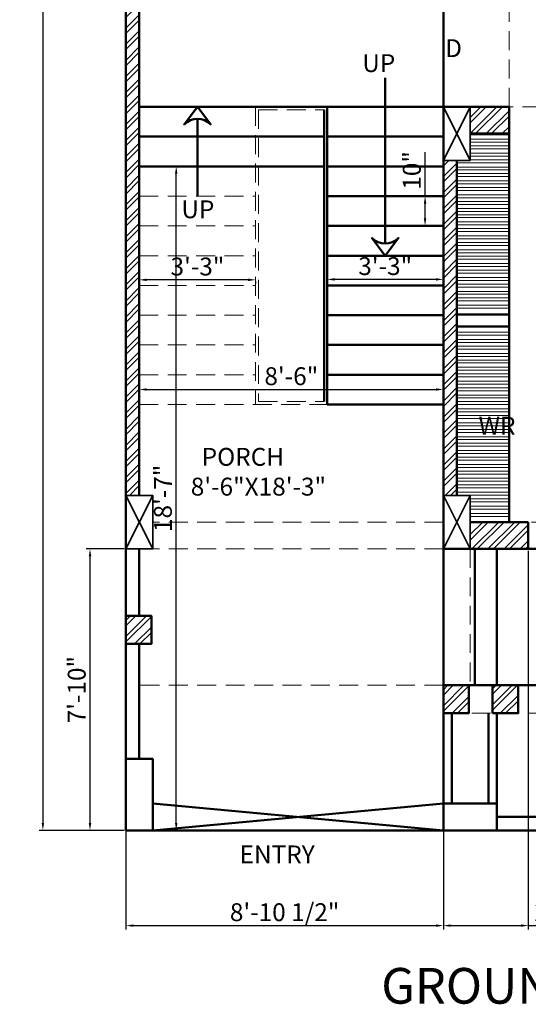
# Model space of a CAD drawing. Units: millimetres. Extents: x 67033 to 68301, y 155969 to 157209.
# Tile 1 of 17: x 67033 to 67203, y 156470 to 156800. Entities that reach past the tile are written whole.
import ezdxf

# ---------------------------------------------------------------- set-up
doc = ezdxf.new("R2010")
doc.units = ezdxf.units.MM
doc.linetypes.add('HIDDEN', pattern=[9.525, 6.35, -3.175])
for name, color, linetype, lineweight in [('A-ANNO-DIMS', 2, 'Continuous', 18), ('A-ANNO-TEXT', 7, 'Continuous', 18), ('A-AREA-IDEN', 3, 'Continuous', 18), ('A-COLS', 3, 'Continuous', 35), ('A-FLOR-OVHD', 1, 'HIDDEN', 18), ('A-FURN', 8, 'Continuous', 18), ('A-WALL', 7, 'Continuous', 50), ('A-WALL-PATT', 8, 'Continuous', 13)]:
    doc.layers.add(name, color=color, linetype=linetype, lineweight=lineweight)
doc.styles.get("Standard").update_dxf_attribs({"font": 'arial.ttf'})
doc.dimstyles.new('ISO-25', dxfattribs={"dimtxt": 6, "dimasz": 2.5, "dimexe": 1.25, "dimexo": 0.625, "dimtad": 1, "dimdec": 0, "dimlunit": 3, "dimtxsty": 'Standard', "dimcen": 2.5, "dimadec": 0, "dimazin": 0, "dimtfac": 1, "dimtdec": 0, "dimtmove": 0, "dimatfit": 3, "dimfxl": 1, "dimarcsym": 0})

# ---------------------------------------------------------------- blocks, each defined once
blk = doc.blocks.new('*D20')
at = {"layer": 'A-ANNO-DIMS', "color": 0, "lineweight": -2, "transparency": 16777216}
for p, q in [((67135.94, 156713.06), (67135.94, 156711.77)), ((67172.44, 156713.02), (67138.44, 156713.02)), ((67174.94, 156713.06), (67174.94, 156711.77))]:
    blk.add_line(p, q, dxfattribs=at)
at = {"layer": 'A-ANNO-DIMS', "color": 0, "transparency": 16777216}
for points in [[(67138.44, 156713.44), (67138.44, 156712.61), (67135.94, 156713.02)], [(67172.44, 156713.44), (67172.44, 156712.61), (67174.94, 156713.02)]]:
    blk.add_solid(points, dxfattribs=at)
at = {"layer": 'Defpoints', "color": 0, "transparency": 16777216}
for p in [(67135.94, 156713.68), (67135.94, 156713.02), (67174.94, 156713.68)]:
    blk.add_point(p, dxfattribs=at)
at = {"layer": 'A-ANNO-DIMS', "color": 0, "transparency": 16777216, "insert": (67155.44, 156716.71), "char_height": 6, "attachment_point": 5}
blk.add_mtext('3\'-3"', dxfattribs=at)
blk = doc.blocks.new('*D21')
at = {"layer": 'A-ANNO-DIMS', "color": 0, "lineweight": -2, "transparency": 16777216}
for p, q in [((67072.94, 156712.4), (67072.94, 156711.63)), ((67109.44, 156712.88), (67075.44, 156712.88)), ((67111.94, 156712.4), (67111.94, 156711.63))]:
    blk.add_line(p, q, dxfattribs=at)
at = {"layer": 'A-ANNO-DIMS', "color": 0, "transparency": 16777216}
for points in [[(67075.44, 156713.29), (67075.44, 156712.46), (67072.94, 156712.88)], [(67109.44, 156713.29), (67109.44, 156712.46), (67111.94, 156712.88)]]:
    blk.add_solid(points, dxfattribs=at)
at = {"layer": 'Defpoints', "color": 0, "transparency": 16777216}
for p in [(67072.94, 156713.02), (67072.94, 156712.88), (67111.94, 156713.02)]:
    blk.add_point(p, dxfattribs=at)
at = {"layer": 'A-ANNO-DIMS', "color": 0, "transparency": 16777216, "insert": (67092.44, 156716.57), "char_height": 6, "attachment_point": 5}
blk.add_mtext('3\'-3"', dxfattribs=at)
blk = doc.blocks.new('*D22')
at = {"layer": 'A-ANNO-DIMS', "color": 0, "lineweight": -2, "transparency": 16777216}
for p, q in [((67072.94, 156676.21), (67072.94, 156677.29)), ((67075.44, 156676.04), (67172.44, 156676.04)), ((67174.94, 156676.21), (67174.94, 156677.29))]:
    blk.add_line(p, q, dxfattribs=at)
at = {"layer": 'A-ANNO-DIMS', "color": 0, "transparency": 16777216}
for points in [[(67075.44, 156676.45), (67075.44, 156675.62), (67072.94, 156676.04)], [(67172.44, 156676.45), (67172.44, 156675.62), (67174.94, 156676.04)]]:
    blk.add_solid(points, dxfattribs=at)
at = {"layer": 'Defpoints', "color": 0, "transparency": 16777216}
for p in [(67072.94, 156675.58), (67174.94, 156676.04), (67174.94, 156675.58)]:
    blk.add_point(p, dxfattribs=at)
at = {"layer": 'A-ANNO-DIMS', "color": 0, "transparency": 16777216, "insert": (67123.94, 156679.73), "char_height": 6, "attachment_point": 5}
blk.add_mtext('8\'-6"', dxfattribs=at)
blk = doc.blocks.new('*D23')
at = {"layer": 'A-ANNO-DIMS', "color": 0, "lineweight": -2, "transparency": 16777216}
for p, q in [((67100.88, 156750.99), (67084.07, 156750.99)), ((67085.32, 156530.49), (67085.32, 156748.49)), ((67100.88, 156527.99), (67084.07, 156527.99))]:
    blk.add_line(p, q, dxfattribs=at)
at = {"layer": 'A-ANNO-DIMS', "color": 0, "transparency": 16777216}
for points in [[(67084.91, 156748.49), (67085.74, 156748.49), (67085.32, 156750.99)], [(67084.91, 156530.49), (67085.74, 156530.49), (67085.32, 156527.99)]]:
    blk.add_solid(points, dxfattribs=at)
at = {"layer": 'Defpoints', "color": 0, "transparency": 16777216}
for p in [(67085.32, 156750.99), (67101.5, 156750.99), (67101.5, 156527.99)]:
    blk.add_point(p, dxfattribs=at)
at = {"layer": 'A-ANNO-DIMS', "color": 0, "transparency": 16777216, "insert": (67081.63, 156639.49), "char_height": 6, "attachment_point": 5, "rotation": 90}
blk.add_mtext('18\'-7"', dxfattribs=at)
blk = doc.blocks.new('*D24')
at = {"layer": 'A-ANNO-DIMS', "color": 0, "lineweight": -2, "transparency": 16777216}
for p, q in [((67168.81, 156740.99), (67168.81, 156755.74)), ((67169.44, 156740.99), (67170.06, 156740.99)), ((67168.81, 156733.49), (67168.81, 156738.49)), ((67169.44, 156730.99), (67170.06, 156730.99))]:
    blk.add_line(p, q, dxfattribs=at)
at = {"layer": 'A-ANNO-DIMS', "color": 0, "transparency": 16777216}
for points in [[(67168.39, 156738.49), (67169.23, 156738.49), (67168.81, 156740.99)], [(67168.39, 156733.49), (67169.23, 156733.49), (67168.81, 156730.99)]]:
    blk.add_solid(points, dxfattribs=at)
at = {"layer": 'Defpoints', "color": 0, "transparency": 16777216}
for p in [(67168.81, 156740.99), (67168.81, 156740.99), (67168.81, 156730.99)]:
    blk.add_point(p, dxfattribs=at)
at = {"layer": 'A-ANNO-DIMS', "color": 0, "transparency": 16777216, "insert": (67165.12, 156749.62), "char_height": 6, "attachment_point": 5, "rotation": 90}
blk.add_mtext('10"', dxfattribs=at)
blk = doc.blocks.new('*D25')
at = {"layer": 'A-ANNO-DIMS', "color": 0, "lineweight": -2, "transparency": 16777216}
for p, q in [((67067.81, 156622.48), (67055.15, 156622.48)), ((67056.4, 156530.49), (67056.4, 156619.98)), ((67067.81, 156527.99), (67055.15, 156527.99))]:
    blk.add_line(p, q, dxfattribs=at)
at = {"layer": 'A-ANNO-DIMS', "color": 0, "transparency": 16777216}
for points in [[(67055.98, 156619.98), (67056.82, 156619.98), (67056.4, 156622.48)], [(67055.98, 156530.49), (67056.82, 156530.49), (67056.4, 156527.99)]]:
    blk.add_solid(points, dxfattribs=at)
at = {"layer": 'Defpoints', "color": 0, "transparency": 16777216}
for p in [(67056.4, 156622.48), (67068.44, 156622.48), (67068.44, 156527.99)]:
    blk.add_point(p, dxfattribs=at)
at = {"layer": 'A-ANNO-DIMS', "color": 0, "transparency": 16777216, "insert": (67052.71, 156575.24), "char_height": 6, "attachment_point": 5, "rotation": 90}
blk.add_mtext('7\'-10"', dxfattribs=at)
blk = doc.blocks.new('*D31')
at = {"layer": 'A-ANNO-DIMS', "color": 0, "lineweight": -2, "transparency": 16777216}
for p, q in [((67067.81, 157136.99), (67039.34, 157136.99)), ((67040.59, 157134.49), (67040.59, 156530.49)), ((67067.81, 156527.99), (67039.34, 156527.99))]:
    blk.add_line(p, q, dxfattribs=at)
at = {"layer": 'A-ANNO-DIMS', "color": 0, "transparency": 16777216}
for points in [[(67040.17, 157134.49), (67041.01, 157134.49), (67040.59, 157136.99)], [(67040.17, 156530.49), (67041.01, 156530.49), (67040.59, 156527.99)]]:
    blk.add_solid(points, dxfattribs=at)
at = {"layer": 'Defpoints', "color": 0, "transparency": 16777216}
for p in [(67068.44, 157136.99), (67040.59, 156527.99), (67068.44, 156527.99)]:
    blk.add_point(p, dxfattribs=at)
at = {"layer": 'A-ANNO-DIMS', "color": 0, "transparency": 16777216, "insert": (67036.9, 156832.49), "char_height": 6, "attachment_point": 5, "rotation": 90}
blk.add_mtext('50\'-9"', dxfattribs=at)
blk = doc.blocks.new('COLUMN-230x460')
for p, q in [((0.44, 17.99), (9.44, -0.01)), ((9.44, 17.99), (0.44, -0.01))]:
    blk.add_line(p, q)
blk.add_lwpolyline([(0.44, 17.99), (9.44, 17.99), (9.44, -0.01), (0.44, -0.01)], close=True)
blk = doc.blocks.new('*D86')
at = {"layer": 'A-ANNO-DIMS', "color": 0, "lineweight": -2, "transparency": 16777216}
for p, q in [((67068.44, 156621.85), (67068.44, 156494.74)), ((67174.94, 156621.87), (67174.94, 156494.74)), ((67070.94, 156495.99), (67172.44, 156495.99))]:
    blk.add_line(p, q, dxfattribs=at)
at = {"layer": 'A-ANNO-DIMS', "color": 0, "transparency": 16777216}
for points in [[(67070.94, 156496.41), (67070.94, 156495.58), (67068.44, 156495.99)], [(67172.44, 156496.41), (67172.44, 156495.58), (67174.94, 156495.99)]]:
    blk.add_solid(points, dxfattribs=at)
at = {"layer": 'Defpoints', "color": 0, "transparency": 16777216}
for p in [(67068.44, 156622.48), (67174.94, 156622.49), (67174.94, 156495.99)]:
    blk.add_point(p, dxfattribs=at)
at = {"layer": 'A-ANNO-DIMS', "color": 0, "transparency": 16777216, "insert": (67121.69, 156499.72), "char_height": 6, "attachment_point": 5}
blk.add_mtext('8\'-10 1/2"', dxfattribs=at)
blk = doc.blocks.new('*D87')
at = {"layer": 'A-ANNO-DIMS', "color": 0, "lineweight": -2, "transparency": 16777216}
for p, q in [((67174.94, 156621.87), (67174.94, 156494.74)), ((67203.44, 156621.87), (67203.44, 156494.74)), ((67177.44, 156495.99), (67200.94, 156495.99)), ((67203.44, 156495.99), (67237.22, 156495.99))]:
    blk.add_line(p, q, dxfattribs=at)
at = {"layer": 'A-ANNO-DIMS', "color": 0, "transparency": 16777216}
for points in [[(67177.44, 156496.41), (67177.44, 156495.58), (67174.94, 156495.99)], [(67200.94, 156496.41), (67200.94, 156495.58), (67203.44, 156495.99)]]:
    blk.add_solid(points, dxfattribs=at)
at = {"layer": 'Defpoints', "color": 0, "transparency": 16777216}
for p in [(67174.94, 156622.49), (67203.44, 156622.49), (67203.44, 156495.99)]:
    blk.add_point(p, dxfattribs=at)
at = {"layer": 'A-ANNO-DIMS', "color": 0, "transparency": 16777216, "insert": (67221.58, 156499.72), "char_height": 6, "attachment_point": 5}
blk.add_mtext('2\'-4 1/2"', dxfattribs=at)

msp = doc.modelspace()

# ---------------------------------------------------------------- hatches: boundary and pattern name
at = {"layer": 'A-WALL-PATT'}
h = msp.add_hatch(dxfattribs=at)
h.set_pattern_fill('ANSI32', color=256, scale=0.4)
h.paths.add_polyline_path([(67072.94, 156817.49), (67068.44, 156817.49), (67068.44, 156640.48), (67072.94, 156640.48)])
h = msp.add_hatch(dxfattribs=at)
h.set_pattern_fill('ANSI32', color=256, scale=0.4)
h.paths.add_polyline_path([(67196.98, 156770.99), (67183.94, 156770.99), (67183.94, 156761.99), (67196.98, 156761.99)])
h = msp.add_hatch(dxfattribs=at)
h.set_pattern_fill('ANSI32', color=256, scale=0.4)
h.paths.add_polyline_path([(67179.44, 156752.99), (67174.94, 156752.99), (67174.94, 156640.48), (67179.44, 156640.48)])
h = msp.add_hatch(dxfattribs=at)
h.set_pattern_fill('ANSI32', color=256, scale=0.4)
h.paths.add_polyline_path([(67203.44, 156631.49), (67183.94, 156631.49), (67183.94, 156622.49), (67203.44, 156622.49)])
h = msp.add_hatch(dxfattribs=at)
h.set_pattern_fill('ANSI32', color=256, scale=0.4)
h.set_pattern_definition([(45, (-106.5, 23.292), (-2.69407684, 2.69407684), []), (45, (-104.704, 23.292), (-2.69407684, 2.69407684), [])])
h.paths.add_polyline_path([(67076.99, 156600.01), (67068.44, 156600.01), (67068.44, 156590.61), (67076.99, 156590.61)])
h = msp.add_hatch(dxfattribs=at)
h.set_pattern_fill('ANSI32', color=256, scale=0.4)
h.paths.add_polyline_path([(67183.49, 156576.72), (67174.94, 156576.72), (67174.94, 156567.32), (67183.49, 156567.32)])
h = msp.add_hatch(dxfattribs=at)
h.set_pattern_fill('ANSI32', color=256, scale=0.4)
h.paths.add_polyline_path([(67200, 156576.72), (67191.45, 156576.72), (67191.45, 156567.32), (67200, 156567.32)])

# ---------------------------------------------------------------- linework, layer by layer
at = {"layer": 'A-FLOR-OVHD'}
for p, q in [((67196.98, 156770.99), (67196.98, 156817.49)), ((67111.94, 156770.99), (67111.94, 156670.99)), ((67236.44, 156770.99), (67196.98, 156770.99)), ((67112.94, 156769.99), (67112.94, 156671.99)), ((67112.94, 156769.99), (67134.94, 156769.99)), ((67072.94, 156740.99), (67111.94, 156740.99)), ((67072.94, 156730.99), (67111.94, 156730.99)), ((67072.94, 156720.99), (67111.94, 156720.99)), ((67072.94, 156710.99), (67111.94, 156710.99)), ((67072.94, 156700.99), (67111.94, 156700.99)), ((67072.94, 156690.99), (67111.94, 156690.99)), ((67072.94, 156680.99), (67111.94, 156680.99)), ((67112.94, 156671.99), (67134.94, 156671.99)), ((67072.94, 156670.99), (67135.94, 156670.99)), ((67174.94, 156631.48), (67077.44, 156631.48)), ((67239.44, 156631.49), (67203.44, 156631.49)), ((67174.94, 156622.48), (67068.44, 156622.48)), ((67183.94, 156622.48), (67183.94, 156576.72)), ((67174.94, 156576.72), (67072.94, 156576.72)), ((67174.94, 156567.32), (67302.44, 156567.32))]:
    msp.add_line(p, q, dxfattribs=at)
at = {"layer": 'A-FURN'}
for p, q in [((67183.94, 156761.54), (67196.98, 156761.54)), ((67183.94, 156760.09), (67196.98, 156760.09)), ((67183.94, 156759.09), (67196.98, 156759.09)), ((67183.94, 156757.87), (67196.98, 156757.87)), ((67183.94, 156756.87), (67196.98, 156756.87)), ((67183.94, 156755.43), (67196.98, 156755.43)), ((67183.94, 156754.43), (67196.98, 156754.43)), ((67179.44, 156752.21), (67196.98, 156752.21)), ((67179.44, 156750.77), (67196.98, 156750.77)), ((67183.83, 156753.21), (67196.98, 156753.21)), ((67179.44, 156749.77), (67196.98, 156749.77)), ((67179.44, 156748.55), (67196.98, 156748.55)), ((67179.44, 156747.55), (67196.98, 156747.55)), ((67179.44, 156746.1), (67196.98, 156746.1)), ((67179.44, 156745.1), (67196.98, 156745.1)), ((67179.44, 156743.88), (67196.98, 156743.88)), ((67179.44, 156742.88), (67196.98, 156742.88)), ((67179.44, 156741.44), (67196.98, 156741.44)), ((67179.44, 156740.44), (67196.98, 156740.44)), ((67179.44, 156739.22), (67196.98, 156739.22)), ((67179.44, 156738.22), (67196.98, 156738.22)), ((67179.44, 156736.78), (67196.98, 156736.78)), ((67179.44, 156735.78), (67196.98, 156735.78)), ((67179.44, 156734.76), (67196.98, 156734.76)), ((67179.44, 156733.76), (67196.98, 156733.76)), ((67179.44, 156732.32), (67196.98, 156732.32)), ((67179.44, 156731.32), (67196.98, 156731.32)), ((67179.44, 156730.1), (67196.98, 156730.1)), ((67179.44, 156729.1), (67196.98, 156729.1)), ((67179.44, 156727.66), (67196.98, 156727.66)), ((67179.44, 156726.66), (67196.98, 156726.66)), ((67179.44, 156725.44), (67196.98, 156725.44)), ((67179.44, 156724.44), (67196.98, 156724.44)), ((67179.44, 156722.99), (67196.98, 156722.99)), ((67179.44, 156721.99), (67196.98, 156721.99)), ((67179.44, 156720.77), (67196.98, 156720.77)), ((67179.44, 156719.77), (67196.98, 156719.77)), ((67179.44, 156718.33), (67196.98, 156718.33)), ((67179.44, 156717.33), (67196.98, 156717.33)), ((67179.44, 156716.11), (67196.98, 156716.11)), ((67179.44, 156715.11), (67196.98, 156715.11)), ((67179.44, 156713.67), (67196.98, 156713.67)), ((67179.44, 156712.67), (67196.98, 156712.67)), ((67179.44, 156711.45), (67196.98, 156711.45)), ((67179.44, 156710.45), (67196.98, 156710.45)), ((67179.44, 156709.01), (67196.98, 156709.01)), ((67179.44, 156708.01), (67196.98, 156708.01)), ((67179.44, 156706.79), (67196.98, 156706.79)), ((67179.44, 156705.79), (67196.98, 156705.79)), ((67179.44, 156704.34), (67196.98, 156704.34)), ((67179.44, 156703.34), (67196.98, 156703.34)), ((67179.44, 156695.28), (67196.98, 156695.28)), ((67179.44, 156694.28), (67196.98, 156694.28)), ((67179.44, 156692.84), (67196.98, 156692.84)), ((67179.44, 156691.84), (67196.98, 156691.84)), ((67179.44, 156690.62), (67196.98, 156690.62)), ((67179.44, 156689.62), (67196.98, 156689.62)), ((67179.44, 156688.17), (67196.98, 156688.17)), ((67179.44, 156687.17), (67196.98, 156687.17)), ((67179.44, 156685.95), (67196.98, 156685.95)), ((67179.44, 156684.95), (67196.98, 156684.95)), ((67179.44, 156683.51), (67196.98, 156683.51)), ((67179.44, 156682.51), (67196.98, 156682.51)), ((67179.44, 156681.29), (67196.98, 156681.29)), ((67179.44, 156680.29), (67196.98, 156680.29)), ((67179.44, 156678.85), (67196.98, 156678.85)), ((67179.44, 156677.85), (67196.98, 156677.85)), ((67179.44, 156676.63), (67196.98, 156676.63)), ((67179.44, 156675.63), (67196.98, 156675.63)), ((67179.44, 156674.19), (67196.98, 156674.19)), ((67179.44, 156673.19), (67196.98, 156673.19)), ((67179.44, 156671.97), (67196.98, 156671.97)), ((67179.44, 156670.97), (67196.98, 156670.97)), ((67179.44, 156669.52), (67196.98, 156669.52)), ((67179.44, 156668.52), (67196.98, 156668.52)), ((67179.44, 156667.3), (67196.98, 156667.3)), ((67179.44, 156666.3), (67196.98, 156666.3)), ((67179.44, 156664.86), (67196.98, 156664.86)), ((67179.44, 156663.86), (67196.98, 156663.86)), ((67179.44, 156662.64), (67196.98, 156662.64)), ((67179.44, 156661.64), (67196.98, 156661.64)), ((67179.44, 156660.2), (67196.98, 156660.2)), ((67179.44, 156659.2), (67196.98, 156659.2)), ((67179.44, 156657.98), (67196.98, 156657.98)), ((67179.44, 156656.98), (67196.98, 156656.98)), ((67179.44, 156655.53), (67196.98, 156655.53)), ((67179.44, 156654.53), (67196.98, 156654.53)), ((67179.44, 156653.31), (67196.98, 156653.31)), ((67179.44, 156652.31), (67196.98, 156652.31)), ((67179.44, 156650.87), (67196.98, 156650.87)), ((67179.44, 156649.87), (67196.98, 156649.87)), ((67179.44, 156648.65), (67196.98, 156648.65)), ((67179.44, 156647.65), (67196.98, 156647.65)), ((67179.44, 156646.21), (67196.98, 156646.21)), ((67179.44, 156645.21), (67196.98, 156645.21)), ((67179.44, 156643.99), (67196.98, 156643.99)), ((67179.44, 156642.99), (67196.98, 156642.99)), ((67179.44, 156641.55), (67196.98, 156641.55)), ((67179.44, 156640.55), (67196.98, 156640.55)), ((67183.94, 156639.33), (67196.98, 156639.33)), ((67183.94, 156638.33), (67196.98, 156638.33)), ((67183.94, 156636.89), (67196.98, 156636.89)), ((67183.94, 156635.89), (67196.98, 156635.89)), ((67183.94, 156634.35), (67196.98, 156634.35)), ((67183.94, 156633.35), (67196.98, 156633.35))]:
    msp.add_line(p, q, dxfattribs=at)
at = {"layer": 'A-WALL'}
for p, q in [((67068.44, 157136.99), (67068.44, 156527.99)), ((67174.94, 156821.99), (67174.94, 156622.49)), ((67072.94, 156817.49), (67072.94, 156640.48)), ((67155.44, 156725.08), (67155.44, 156780.67)), ((67072.94, 156770.99), (67174.94, 156770.99)), ((67135.94, 156770.99), (67135.94, 156670.99)), ((67174.94, 156770.99), (67196.98, 156770.99)), ((67196.98, 156770.99), (67196.98, 156631.49)), ((67134.94, 156769.99), (67134.94, 156671.99)), ((67092.44, 156740.99), (67092.44, 156766.9)), ((67072.94, 156760.99), (67134.94, 156760.99)), ((67135.94, 156760.99), (67174.94, 156760.99)), ((67183.94, 156761.99), (67196.98, 156761.99)), ((67072.94, 156750.99), (67134.94, 156750.99)), ((67135.94, 156750.99), (67174.94, 156750.99)), ((67179.44, 156752.99), (67179.44, 156640.48)), ((67135.94, 156740.99), (67174.94, 156740.99)), ((67135.94, 156730.99), (67174.94, 156730.99)), ((67135.94, 156720.99), (67174.94, 156720.99)), ((67135.94, 156710.99), (67174.94, 156710.99)), ((67135.94, 156700.99), (67174.94, 156700.99)), ((67196.98, 156701.24), (67179.44, 156701.24)), ((67196.98, 156697.24), (67179.44, 156697.24)), ((67135.94, 156690.99), (67174.94, 156690.99)), ((67135.94, 156680.99), (67174.94, 156680.99)), ((67135.94, 156670.99), (67174.94, 156670.99)), ((67183.94, 156631.49), (67203.44, 156631.49)), ((67203.44, 156631.49), (67203.44, 156622.49)), ((67072.94, 156622.48), (67072.94, 156600.01)), ((67174.94, 156622.49), (67203.44, 156622.49)), ((67174.94, 156622.48), (67174.94, 156527.99)), ((67185.55, 156622.49), (67185.55, 156576.72)), ((67192.94, 156576.72), (67192.94, 156622.49)), ((67203.44, 156622.49), (67239.44, 156622.49)), ((67072.94, 156590.61), (67072.94, 156551.99)), ((67174.94, 156576.72), (67302.44, 156576.72)), ((67177.84, 156567.32), (67177.84, 156536.99)), ((67190.04, 156567.32), (67190.04, 156536.99)), ((67192.94, 156536.99), (67192.94, 156567.32)), ((67174.94, 156536.99), (67077.44, 156527.99)), ((67174.94, 156527.99), (67077.44, 156536.99)), ((67192.94, 156532.49), (67407.44, 156532.49)), ((67068.44, 156527.99), (67407.44, 156527.99))]:
    msp.add_line(p, q, dxfattribs=at)
for points in [[(67092.44, 156770.99), (67096.9, 156765.06, 0.414166), (67087.98, 156765.06)], [(67155.44, 156720.99), (67150.98, 156726.93, 0.414166), (67159.9, 156726.93)]]:
    msp.add_lwpolyline(points, format="xyb", close=True, dxfattribs=at)
for points in [[(67068.44, 156590.61), (67076.99, 156590.61), (67076.99, 156600.01), (67068.44, 156600.01)], [(67174.94, 156567.32), (67183.49, 156567.32), (67183.49, 156576.72), (67174.94, 156576.72)], [(67191.45, 156567.32), (67200, 156567.32), (67200, 156576.72), (67191.45, 156576.72)], [(67068.44, 156527.99), (67077.44, 156527.99), (67077.44, 156551.99), (67068.44, 156551.99)], [(67174.94, 156527.99), (67192.94, 156527.99), (67192.94, 156536.99), (67174.94, 156536.99)]]:
    msp.add_lwpolyline(points, close=True, dxfattribs=at)

# ---------------------------------------------------------------- block references
at = {"layer": 'A-COLS'}
for p in [(67174.5, 156753), (67068, 156622.49)]:
    msp.add_blockref('COLUMN-230x460', p, dxfattribs=at)
at = {"layer": 'A-COLS', "extrusion": (0, 0, -1), "zscale": -1, "rotation": 180.0076170266062}
msp.add_blockref('COLUMN-230x460', (-67174.5, 156640.48), dxfattribs=at)

# ---------------------------------------------------------------- texts
at = {"layer": 'A-ANNO-TEXT', "attachment_point": 1}
for s, width, insert, char_height in [('   D', 19.5287, (67170.06, 156793.68), 6), (' UP', 19.5287, (67145.89, 156788.65), 6), (' UP', 19.5287, (67085.21, 156739.56), 6), ('   WR', 19.5287, (67181.25, 156666.88), 6), ('GROUND FLOOR PLAN', 203.6887, (67154.11, 156481.77), 12)]:
    msp.add_mtext_dynamic_manual_height_columns(s, width=width, gutter_width=12.5, heights=[0], dxfattribs=dict(at, insert=insert, char_height=char_height))
at = {"layer": 'A-AREA-IDEN', "char_height": 6, "attachment_point": 1}
for s, width, insert in [('       PORCH\\P     8\'-6"X18\'-3"', 75.351, (67081.03, 156656.42)), ('    ENTRY', 59.4046, (67099.26, 156522.9))]:
    msp.add_mtext_dynamic_manual_height_columns(s, width=width, gutter_width=12.5, heights=[0], dxfattribs=dict(at, insert=insert))

# ---------------------------------------------------------------- dimensions: what is measured, and where the dimension line sits
at = {"layer": 'A-ANNO-DIMS'}
for base, p1, p2, picture, middle in [((67040.59, 156527.99), (67068.44, 157136.99), (67068.44, 156527.99), '*D31', (67036.9, 156832.49)), ((67168.81, 156740.99), (67168.81, 156730.99), (67168.81, 156740.99), '*D24', (67165.12, 156749.62)), ((67085.32, 156750.99), (67101.5, 156527.99), (67101.5, 156750.99), '*D23', (67081.63, 156639.49)), ((67056.4, 156622.48), (67068.44, 156527.99), (67068.44, 156622.48), '*D25', (67052.71, 156575.24))]:
    dim = msp.add_linear_dim(base=base, p1=p1, p2=p2, angle=90, dimstyle='ISO-25', override={"dimclrd": 0, "dimclre": 0, "dimclrt": 0}, dxfattribs=at)
    dim.commit()
    dim.dimension.update_dxf_attribs({"geometry": picture, "text_midpoint": middle})
for base, p1, p2, override, picture, middle in [((67135.94, 156713.02), (67174.94, 156713.68), (67135.94, 156713.68), {"dimclrd": 0, "dimclre": 0, "dimclrt": 0}, '*D20', (67155.44, 156716.71)), ((67072.94, 156712.88), (67111.94, 156713.02), (67072.94, 156713.02), {"dimclrd": 0, "dimclre": 0, "dimclrt": 0}, '*D21', (67092.44, 156716.57)), ((67174.94, 156676.04), (67072.94, 156675.58), (67174.94, 156675.58), {"dimclrd": 0, "dimclre": 0, "dimclrt": 0}, '*D22', (67123.94, 156679.73)), ((67174.94, 156495.99), (67068.44, 156622.48), (67174.94, 156622.49), {"dimdec": 1, "dimlfac": 1, "dimrnd": 0, "dimzin": 1, "dimdsep": 46, "dimlunit": 4, "dimfrac": 2}, '*D86', (67121.69, 156499.72)), ((67203.44, 156495.99), (67174.94, 156622.49), (67203.44, 156622.49), {"dimdec": 1, "dimlfac": 1, "dimrnd": 0, "dimzin": 1, "dimdsep": 46, "dimlunit": 4, "dimfrac": 2}, '*D87', (67221.58, 156499.72))]:
    dim = msp.add_linear_dim(base=base, p1=p1, p2=p2, dimstyle='ISO-25', override=override, dxfattribs=at)
    dim.commit()
    dim.dimension.update_dxf_attribs({"geometry": picture, "text_midpoint": middle})

doc.saveas('drawing.dxf')
